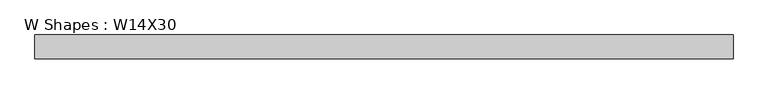
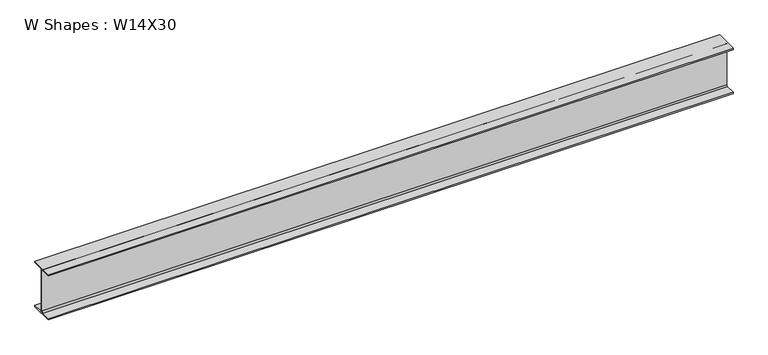
"""IFC4 building model written with IfcOpenShell, lengths in millimetres: beam geometry, W Shapes : W14X30."""

from ifc_helpers import new_model, si_unit, point, frame, frame_2d, origin, place, context, project, spatial, polyline, circle_curve, trimmed, segment, composite_curve, outline, extrude, source, transform, mapped, element, save


def w_shapes_w14x30_920474df(model_context):
    return source(origin(), model_context, "Body", "SweptSolid", [
        extrude(outline(composite_curve([segment(polyline([(85.471, -165.481), (85.471, -175.26), (-85.471, -175.26), (-85.471, -165.481), (-13.589, -165.481)]), True, "CONTINUOUS"), segment(trimmed(circle_curve(frame_2d((-13.589, -155.321)), 10.16), [point((-13.589, -165.481))], [point((-3.429, -155.321))], True, "CARTESIAN"), True, "CONTINUOUS"), segment(polyline([(-3.429, -155.321), (-3.429, 155.321)]), True, "CONTINUOUS"), segment(trimmed(circle_curve(frame_2d((-13.589, 155.321)), 10.16), [point((-3.429, 155.321))], [point((-13.589, 165.481))], True, "CARTESIAN"), True, "CONTINUOUS"), segment(polyline([(-13.589, 165.481), (-85.471, 165.481), (-85.471, 175.26), (85.471, 175.26), (85.471, 165.481), (13.589, 165.481)]), True, "CONTINUOUS"), segment(trimmed(circle_curve(frame_2d((13.589, 155.321)), 10.16), [point((13.589, 165.481))], [point((3.429, 155.321))], True, "CARTESIAN"), True, "CONTINUOUS"), segment(polyline([(3.429, 155.321), (3.429, -155.321)]), True, "CONTINUOUS"), segment(trimmed(circle_curve(frame_2d((13.589, -155.321)), 10.16), [point((3.429, -155.321))], [point((13.589, -165.481))], True, "CARTESIAN"), True, "CONTINUOUS"), segment(polyline([(13.589, -165.481), (85.471, -165.481)]), True, "CONTINUOUS")], self_intersect=False)), frame((-2500.0, 0.0, 0.0), z_axis=(1.0, 0.0, 0.0), x_axis=(0.0, 1.0, 0.0)), (0.0, 0.0, 1.0), 5000.0),
    ])


if __name__ == "__main__":
    model = new_model("IFC4")
    model_context = context("Model", 3, world=origin())
    ifc_project = project(units=[si_unit("LENGTHUNIT", "METRE", prefix="MILLI")], contexts=[model_context])
    site = spatial("IfcSite", under=ifc_project)
    building = spatial("IfcBuilding", under=site)
    placement = place(None, origin())
    w_shapes_w14x30_shape = w_shapes_w14x30_920474df(model_context)
    element("IfcBeam", 1, ObjectType="W Shapes : W14X30", at=placement, inside=building, context=model_context, shape_type="MappedRepresentation", body=[
        mapped(w_shapes_w14x30_shape, transform((0.0, 0.0, 0.0), x_axis=(1.0, 0.0, 0.0), y_axis=(0.0, 1.0, 0.0), z_axis=(0.0, 0.0, 1.0))),
    ])
    save(model, "model.ifc")

# Revit data of these elements
# Type "W Shapes : W14X30"
#   Section Name Key = "W14X30"
#   Width = 6.730"
#   Web Thickness = 0.270"
#   Web Fillet = 0.400"
#   Warping Constant = 887.00 in⁶
#   Torsional Moment of Inertia = 0.38 in⁴
#   Section Area = 8.85 in²
#   Plastic Modulus weak axis = 8.99 in³
#   Plastic Modulus strong axis = 47.30 in³
#   Perimeter = 4.441 ft²/ft
#   Nominal Weight = 30.00 lbf/ft
#   Moment of Inertia weak axis = 19.60 in⁴
#   Moment of Inertia strong axis = 291.00 in⁴
#   Height = 13.800"
#   Flange Thickness = 0.385"
#   Elastic Modulus weak axis = 5.82 in³
#   Elastic Modulus strong axis = 42.00 in³
#   Clear Web Height = 0' - 11 5/8"
#   Centroid Vertical = 6.900"
#   Centroid Horizontal = 3.365"
#   Bolt Spacing = 0' - 3 1/2"
#   Length [instance default] = 1524 mm
#   Structural Material [instance default] = Steel ASTM A992
#   Principal Axes Angle = 0
# Element 1 (IfcBeam, "W Shapes : W14X30")
#   Length = 5000 mm
#   Materials on its faces: "Steel ASTM A992"
# Materials
#   "Steel ASTM A992": class "Metal", colour RGB 199 199 199, transparency 0, Description = "Structural steel 50ksi", Cost = 0
